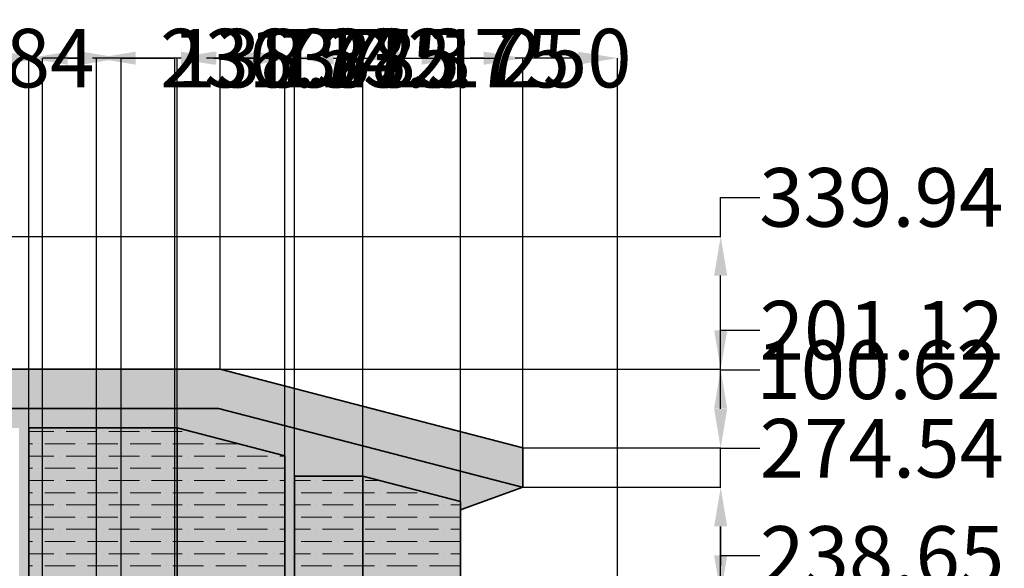
# Model space of a CAD drawing. Units: millimetres. Extents: x -504 to 6314, y 1290 to 4335.
# Tile 9 of 9: x 3796 to 6314, y 2932 to 4335. Entities that reach past the tile are written whole.
import ezdxf

# ---------------------------------------------------------------- set-up
doc = ezdxf.new("R2010")
doc.units = ezdxf.units.MM
doc.header["$MEASUREMENT"] = 0
for name, color, linetype, lineweight in [('A-ANNO-DIMS', 2, 'Continuous', 18), ('A-ELEV', 7, 'Continuous', 35), ('A-ELEV-PATT', 8, 'Continuous', 13)]:
    doc.layers.add(name, color=color, linetype=linetype, lineweight=lineweight)
doc.styles.get("Standard").update_dxf_attribs({"font": 'arial.ttf'})
doc.dimstyles.get("Standard").update_dxf_attribs({"dimtxt": 150, "dimasz": 100, "dimexe": 0.18, "dimexo": 0.0625, "dimgap": 0.09, "dimtad": 0, "dimtih": 1, "dimtoh": 1, "dimdec": 0, "dimzin": 0, "dimdsep": 46, "dimtxsty": 'Standard', "dimcen": 0.09, "dimadec": 0, "dimazin": 0, "dimtfac": 1, "dimtdec": 0, "dimtofl": 0, "dimtmove": 0, "dimatfit": 3, "dimfxl": 1, "dimtolj": 1, "dimtzin": 0, "dimarcsym": 0})

# ---------------------------------------------------------------- blocks, each defined once
blk = doc.blocks.new('*D22')
at = {"layer": 'A-ANNO-DIMS', "color": 0, "lineweight": -2, "transparency": 16777216}
for p, q in [((3324.5, 3780.7), (3324.5, 4237)), ((3424.5, 4236.8), (3651, 4236.8)), ((4208.6, 4236.8), (3982, 4236.8)), ((4308.6, 3440.7), (4308.6, 4237))]:
    blk.add_line(p, q, dxfattribs=at)
at = {"layer": 'A-ANNO-DIMS', "color": 0, "transparency": 16777216}
for points in [[(3424.5, 4253.4), (3424.5, 4220.1), (3324.5, 4236.8)], [(4208.6, 4253.4), (4208.6, 4220.1), (4308.6, 4236.8)]]:
    blk.add_solid(points, dxfattribs=at)
at = {"layer": 'Defpoints', "color": 0, "transparency": 16777216}
for p in [(4308.6, 4236.8), (3324.5, 3780.6), (4308.6, 3440.7)]:
    blk.add_point(p, dxfattribs=at)
at = {"layer": 'A-ANNO-DIMS', "color": 0, "transparency": 16777216, "insert": (3816.5, 4236.8), "char_height": 150, "attachment_point": 5}
blk.add_mtext('\\A1;984', dxfattribs=at)
blk = doc.blocks.new('*D23')
at = {"layer": 'A-ANNO-DIMS', "color": 0, "lineweight": -2, "transparency": 16777216}
for p, q in [((4308.6, 3440.7), (4308.6, 4237)), ((4408.6, 4236.8), (4443.2, 4236.8)), ((4982.9, 4236.8), (4948.3, 4236.8)), ((5082.9, 3239.6), (5082.9, 4237))]:
    blk.add_line(p, q, dxfattribs=at)
at = {"layer": 'A-ANNO-DIMS', "color": 0, "transparency": 16777216}
for points in [[(4408.6, 4253.4), (4408.6, 4220.1), (4308.6, 4236.8)], [(4982.9, 4253.4), (4982.9, 4220.1), (5082.9, 4236.8)]]:
    blk.add_solid(points, dxfattribs=at)
at = {"layer": 'Defpoints', "color": 0, "transparency": 16777216}
for p in [(5082.9, 4236.8), (4308.6, 3440.7), (5082.9, 3239.6)]:
    blk.add_point(p, dxfattribs=at)
at = {"layer": 'A-ANNO-DIMS', "color": 0, "transparency": 16777216, "insert": (4695.7, 4236.8), "char_height": 150, "attachment_point": 5}
blk.add_mtext('\\A1;774.3', dxfattribs=at)
blk = doc.blocks.new('*D24')
at = {"layer": 'A-ANNO-DIMS', "color": 0, "lineweight": -2, "transparency": 16777216}
for p, q in [((5588.8, 3780.6), (5588.8, 3880.6)), ((5588.8, 3880.6), (5688.8, 3880.6)), ((3324.5, 3780.6), (5589, 3780.6)), ((5588.8, 3540.7), (5588.8, 3680.6)), ((4308.6, 3440.7), (5589, 3440.7))]:
    blk.add_line(p, q, dxfattribs=at)
at = {"layer": 'A-ANNO-DIMS', "color": 0, "transparency": 16777216}
for points in [[(5572.1, 3680.6), (5605.5, 3680.6), (5588.8, 3780.6)], [(5572.1, 3540.7), (5605.5, 3540.7), (5588.8, 3440.7)]]:
    blk.add_solid(points, dxfattribs=at)
at = {"layer": 'Defpoints', "color": 0, "transparency": 16777216}
for p in [(3324.5, 3780.6), (5588.8, 3780.6), (4308.6, 3440.7)]:
    blk.add_point(p, dxfattribs=at)
at = {"layer": 'A-ANNO-DIMS', "color": 0, "transparency": 16777216, "insert": (5999.9, 3880.6), "char_height": 150, "attachment_point": 5}
blk.add_mtext('\\A1;339.94', dxfattribs=at)
blk = doc.blocks.new('*D25')
at = {"layer": 'A-ANNO-DIMS', "color": 0, "lineweight": -2, "transparency": 16777216}
for p, q in [((5588.8, 3339.6), (5588.8, 3439.6)), ((5588.8, 3439.6), (5688.8, 3439.6)), ((5082.9, 3239.6), (5589, 3239.6)), ((5081.2, 3138.9), (5589, 3138.9)), ((5588.8, 3038.9), (5588.8, 2938.9))]:
    blk.add_line(p, q, dxfattribs=at)
at = {"layer": 'A-ANNO-DIMS', "color": 0, "transparency": 16777216}
for points in [[(5572.1, 3339.6), (5605.5, 3339.6), (5588.8, 3239.6)], [(5572.1, 3038.9), (5605.5, 3038.9), (5588.8, 3138.9)]]:
    blk.add_solid(points, dxfattribs=at)
at = {"layer": 'Defpoints', "color": 0, "transparency": 16777216}
for p in [(5082.9, 3239.6), (5588.8, 3239.6), (5081.2, 3138.9)]:
    blk.add_point(p, dxfattribs=at)
at = {"layer": 'A-ANNO-DIMS', "color": 0, "transparency": 16777216, "insert": (5992.4, 3439.6), "char_height": 150, "attachment_point": 5}
blk.add_mtext('\\A1;100.62', dxfattribs=at)
blk = doc.blocks.new('*D26')
at = {"layer": 'A-ANNO-DIMS', "color": 0, "lineweight": -2, "transparency": 16777216}
for p, q in [((5588.8, 3440.7), (5588.8, 3540.7)), ((5588.8, 3540.7), (5688.8, 3540.7)), ((4308.6, 3440.7), (5589, 3440.7)), ((5588.8, 3339.6), (5588.8, 3340.7)), ((5082.9, 3239.6), (5589, 3239.6))]:
    blk.add_line(p, q, dxfattribs=at)
at = {"layer": 'A-ANNO-DIMS', "color": 0, "transparency": 16777216}
for points in [[(5572.1, 3340.7), (5605.5, 3340.7), (5588.8, 3440.7)], [(5572.1, 3339.6), (5605.5, 3339.6), (5588.8, 3239.6)]]:
    blk.add_solid(points, dxfattribs=at)
at = {"layer": 'Defpoints', "color": 0, "transparency": 16777216}
for p in [(4308.6, 3440.7), (5588.8, 3440.7), (5082.9, 3239.6)]:
    blk.add_point(p, dxfattribs=at)
at = {"layer": 'A-ANNO-DIMS', "color": 0, "transparency": 16777216, "insert": (6000.8, 3540.7), "char_height": 150, "attachment_point": 5}
blk.add_mtext('\\A1;201.12', dxfattribs=at)
blk = doc.blocks.new('*D27')
at = {"layer": 'A-ANNO-DIMS', "color": 0, "lineweight": -2, "transparency": 16777216}
for p, q in [((5588.8, 3138.9), (5588.8, 3238.9)), ((5588.8, 3238.9), (5688.8, 3238.9)), ((5081.2, 3138.9), (5589, 3138.9)), ((5588.8, 2964.4), (5588.8, 3038.9)), ((4489, 2864.4), (5589, 2864.4))]:
    blk.add_line(p, q, dxfattribs=at)
at = {"layer": 'A-ANNO-DIMS', "color": 0, "transparency": 16777216}
for points in [[(5572.1, 3038.9), (5605.5, 3038.9), (5588.8, 3138.9)], [(5572.1, 2964.4), (5605.5, 2964.4), (5588.8, 2864.4)]]:
    blk.add_solid(points, dxfattribs=at)
at = {"layer": 'Defpoints', "color": 0, "transparency": 16777216}
for p in [(5081.2, 3138.9), (5588.8, 3138.9), (4489, 2864.4)]:
    blk.add_point(p, dxfattribs=at)
at = {"layer": 'A-ANNO-DIMS', "color": 0, "transparency": 16777216, "insert": (6001.2, 3238.9), "char_height": 150, "attachment_point": 5}
blk.add_mtext('\\A1;274.54', dxfattribs=at)
blk = doc.blocks.new('*D28')
at = {"layer": 'A-ANNO-DIMS', "color": 0, "lineweight": -2, "transparency": 16777216}
for p, q in [((-191.2, 3540.7), (-191.2, 3640.7)), ((-191.2, 3640.7), (-91.2, 3640.7)), ((4308.5, 3440.7), (-191.3, 3440.7)), ((4304.4, 3340.7), (-191.3, 3340.7)), ((-191.2, 3240.7), (-191.2, 3140.7))]:
    blk.add_line(p, q, dxfattribs=at)
at = {"layer": 'A-ANNO-DIMS', "color": 0, "transparency": 16777216}
for points in [[(-207.8, 3540.7), (-174.5, 3540.7), (-191.2, 3440.7)], [(-207.8, 3240.7), (-174.5, 3240.7), (-191.2, 3340.7)]]:
    blk.add_solid(points, dxfattribs=at)
at = {"layer": 'Defpoints', "color": 0, "transparency": 16777216}
for p in [(-191.2, 3440.7), (4308.6, 3440.7), (4304.5, 3340.7)]:
    blk.add_point(p, dxfattribs=at)
at = {"layer": 'A-ANNO-DIMS', "color": 0, "transparency": 16777216, "insert": (67.3, 3640.7), "char_height": 150, "attachment_point": 5}
blk.add_mtext('\\A1;100', dxfattribs=at)
blk = doc.blocks.new('*D29')
at = {"layer": 'A-ANNO-DIMS', "color": 0, "lineweight": -2, "transparency": 16777216}
for p, q in [((5588.8, 2864.4), (5588.8, 2964.4)), ((5588.8, 2964.4), (5688.8, 2964.4)), ((4489, 2864.4), (5589, 2864.4)), ((5588.8, 2725.8), (5588.8, 2764.4)), ((4260.1, 2625.8), (5589, 2625.8))]:
    blk.add_line(p, q, dxfattribs=at)
at = {"layer": 'A-ANNO-DIMS', "color": 0, "transparency": 16777216}
for points in [[(5572.1, 2764.4), (5605.5, 2764.4), (5588.8, 2864.4)], [(5572.1, 2725.8), (5605.5, 2725.8), (5588.8, 2625.8)]]:
    blk.add_solid(points, dxfattribs=at)
at = {"layer": 'Defpoints', "color": 0, "transparency": 16777216}
for p in [(4489, 2864.4), (5588.8, 2864.4), (4260, 2625.8)]:
    blk.add_point(p, dxfattribs=at)
at = {"layer": 'A-ANNO-DIMS', "color": 0, "transparency": 16777216, "insert": (6002.1, 2964.4), "char_height": 150, "attachment_point": 5}
blk.add_mtext('\\A1;238.65', dxfattribs=at)
blk = doc.blocks.new('*D44')
at = {"layer": 'A-ANNO-DIMS', "color": 0, "lineweight": -2, "transparency": 16777216}
for p, q in [((4198.6, 3290.7), (4198.6, 4237)), ((4298.6, 4236.8), (4373.6, 4236.8)), ((4473.6, 3219.3), (4473.6, 4237)), ((4473.6, 4236.8), (4573.6, 4236.8))]:
    blk.add_line(p, q, dxfattribs=at)
at = {"layer": 'A-ANNO-DIMS', "color": 0, "transparency": 16777216}
for points in [[(4298.6, 4253.4), (4298.6, 4220.1), (4198.6, 4236.8)], [(4373.6, 4253.4), (4373.6, 4220.1), (4473.6, 4236.8)]]:
    blk.add_solid(points, dxfattribs=at)
at = {"layer": 'Defpoints', "color": 0, "transparency": 16777216}
for p in [(4473.6, 4236.8), (4198.6, 3290.7), (4473.6, 3219.3)]:
    blk.add_point(p, dxfattribs=at)
at = {"layer": 'A-ANNO-DIMS', "color": 0, "transparency": 16777216, "insert": (4741.3, 4236.8), "char_height": 150, "attachment_point": 5}
blk.add_mtext('\\A1;275', dxfattribs=at)
blk = doc.blocks.new('*D45')
at = {"layer": 'A-ANNO-DIMS', "color": 0, "lineweight": -2, "transparency": 16777216}
for p, q in [((4373.6, 4236.8), (4273.6, 4236.8)), ((4473.6, 3219.3), (4473.6, 4237)), ((4498.6, 3167.4), (4498.6, 4237)), ((4598.6, 4236.8), (4698.6, 4236.8))]:
    blk.add_line(p, q, dxfattribs=at)
at = {"layer": 'A-ANNO-DIMS', "color": 0, "transparency": 16777216}
for points in [[(4373.6, 4253.4), (4373.6, 4220.1), (4473.6, 4236.8)], [(4598.6, 4253.4), (4598.6, 4220.1), (4498.6, 4236.8)]]:
    blk.add_solid(points, dxfattribs=at)
at = {"layer": 'Defpoints', "color": 0, "transparency": 16777216}
for p in [(4498.6, 4236.8), (4473.6, 3219.3), (4498.6, 3167.3)]:
    blk.add_point(p, dxfattribs=at)
at = {"layer": 'A-ANNO-DIMS', "color": 0, "transparency": 16777216, "insert": (4808, 4236.8), "char_height": 150, "attachment_point": 5}
blk.add_mtext('\\A1;25', dxfattribs=at)
blk = doc.blocks.new('*D46')
at = {"layer": 'A-ANNO-DIMS', "color": 0, "lineweight": -2, "transparency": 16777216}
for p, q in [((4398.6, 4236.8), (4298.6, 4236.8)), ((4498.6, 3167.4), (4498.6, 4237)), ((4673.6, 3167.4), (4673.6, 4237)), ((4773.6, 4236.8), (4873.6, 4236.8))]:
    blk.add_line(p, q, dxfattribs=at)
at = {"layer": 'A-ANNO-DIMS', "color": 0, "transparency": 16777216}
for points in [[(4398.6, 4253.4), (4398.6, 4220.1), (4498.6, 4236.8)], [(4773.6, 4253.4), (4773.6, 4220.1), (4673.6, 4236.8)]]:
    blk.add_solid(points, dxfattribs=at)
at = {"layer": 'Defpoints', "color": 0, "transparency": 16777216}
for p in [(4673.6, 4236.8), (4498.6, 3167.3), (4673.6, 3167.3)]:
    blk.add_point(p, dxfattribs=at)
at = {"layer": 'A-ANNO-DIMS', "color": 0, "transparency": 16777216, "insert": (5032.9, 4236.8), "char_height": 150, "attachment_point": 5}
blk.add_mtext('\\A1;175', dxfattribs=at)
blk = doc.blocks.new('*D47')
at = {"layer": 'A-ANNO-DIMS', "color": 0, "lineweight": -2, "transparency": 16777216}
for p, q in [((4673.6, 3167.4), (4673.6, 4237)), ((4773.6, 4236.8), (4823.6, 4236.8)), ((4923.6, 3102.4), (4923.6, 4237)), ((4923.6, 4236.8), (5023.6, 4236.8))]:
    blk.add_line(p, q, dxfattribs=at)
at = {"layer": 'A-ANNO-DIMS', "color": 0, "transparency": 16777216}
for points in [[(4773.6, 4253.4), (4773.6, 4220.1), (4673.6, 4236.8)], [(4823.6, 4253.4), (4823.6, 4220.1), (4923.6, 4236.8)]]:
    blk.add_solid(points, dxfattribs=at)
at = {"layer": 'Defpoints', "color": 0, "transparency": 16777216}
for p in [(4923.6, 4236.8), (4673.6, 3167.3), (4923.6, 3102.4)]:
    blk.add_point(p, dxfattribs=at)
at = {"layer": 'A-ANNO-DIMS', "color": 0, "transparency": 16777216, "insert": (5190.5, 4236.8), "char_height": 150, "attachment_point": 5}
blk.add_mtext('\\A1;250', dxfattribs=at)
blk = doc.blocks.new('*D60')
at = {"layer": 'A-ANNO-DIMS', "color": 0, "lineweight": -2, "transparency": 16777216}
for p, q in [((3818.6, 2525.8), (3818.6, 4237)), ((3918.6, 4236.8), (3955.1, 4236.8)), ((4055.1, 2525.8), (4055.1, 4237)), ((4055.1, 4236.8), (4155.1, 4236.8))]:
    blk.add_line(p, q, dxfattribs=at)
at = {"layer": 'A-ANNO-DIMS', "color": 0, "transparency": 16777216}
for points in [[(3918.6, 4253.4), (3918.6, 4220.1), (3818.6, 4236.8)], [(3955.1, 4253.4), (3955.1, 4220.1), (4055.1, 4236.8)]]:
    blk.add_solid(points, dxfattribs=at)
at = {"layer": 'Defpoints', "color": 0, "transparency": 16777216}
for p in [(4055.1, 4236.8), (3818.6, 2525.8), (4055.1, 2525.8)]:
    blk.add_point(p, dxfattribs=at)
at = {"layer": 'A-ANNO-DIMS', "color": 0, "transparency": 16777216, "insert": (4410.2, 4236.8), "char_height": 150, "attachment_point": 5}
blk.add_mtext('\\A1;236.5', dxfattribs=at)
blk = doc.blocks.new('*D61')
at = {"layer": 'A-ANNO-DIMS', "color": 0, "lineweight": -2, "transparency": 16777216}
for p, q in [((3955.1, 4236.8), (3855.1, 4236.8)), ((4055.1, 2525.8), (4055.1, 4237)), ((4192.1, 2525.8), (4192.1, 4237)), ((4292.1, 4236.8), (4392.1, 4236.8))]:
    blk.add_line(p, q, dxfattribs=at)
at = {"layer": 'A-ANNO-DIMS', "color": 0, "transparency": 16777216}
for points in [[(3955.1, 4253.4), (3955.1, 4220.1), (4055.1, 4236.8)], [(4292.1, 4253.4), (4292.1, 4220.1), (4192.1, 4236.8)]]:
    blk.add_solid(points, dxfattribs=at)
at = {"layer": 'Defpoints', "color": 0, "transparency": 16777216}
for p in [(4192.1, 4236.8), (4055.1, 2525.8), (4192.1, 2525.8)]:
    blk.add_point(p, dxfattribs=at)
at = {"layer": 'A-ANNO-DIMS', "color": 0, "transparency": 16777216, "insert": (4550.9, 4236.8), "char_height": 150, "attachment_point": 5}
blk.add_mtext('\\A1;137', dxfattribs=at)
blk = doc.blocks.new('*D62')
at = {"layer": 'A-ANNO-DIMS', "color": 0, "lineweight": -2, "transparency": 16777216}
for p, q in [((4192.1, 2525.8), (4192.1, 4237)), ((4292.1, 4236.8), (4454.1, 4236.8)), ((5224.8, 4236.8), (5062.8, 4236.8)), ((5324.8, 2338.9), (5324.8, 4237))]:
    blk.add_line(p, q, dxfattribs=at)
at = {"layer": 'A-ANNO-DIMS', "color": 0, "transparency": 16777216}
for points in [[(4292.1, 4253.4), (4292.1, 4220.1), (4192.1, 4236.8)], [(5224.8, 4253.4), (5224.8, 4220.1), (5324.8, 4236.8)]]:
    blk.add_solid(points, dxfattribs=at)
at = {"layer": 'Defpoints', "color": 0, "transparency": 16777216}
for p in [(5324.8, 4236.8), (4192.1, 2525.8), (5324.8, 2338.8)]:
    blk.add_point(p, dxfattribs=at)
at = {"layer": 'A-ANNO-DIMS', "color": 0, "transparency": 16777216, "insert": (4758.5, 4236.8), "char_height": 150, "attachment_point": 5}
blk.add_mtext('\\A1;1132.7', dxfattribs=at)
blk = doc.blocks.new('*D66')
at = {"layer": 'A-ANNO-DIMS', "color": 0, "lineweight": -2, "transparency": 16777216}
for p, q in [((3753.7, 4236.8), (3653.7, 4236.8)), ((3853.7, 1932.9), (3853.7, 4237)), ((3992.1, 1982.9), (3992.1, 4237)), ((4092.1, 4236.8), (4192.1, 4236.8))]:
    blk.add_line(p, q, dxfattribs=at)
at = {"layer": 'A-ANNO-DIMS', "color": 0, "transparency": 16777216}
for points in [[(3753.7, 4253.4), (3753.7, 4220.1), (3853.7, 4236.8)], [(4092.1, 4253.4), (4092.1, 4220.1), (3992.1, 4236.8)]]:
    blk.add_solid(points, dxfattribs=at)
at = {"layer": 'Defpoints', "color": 0, "transparency": 16777216}
for p in [(3992.1, 4236.8), (3992.1, 1982.8), (3853.7, 1932.8)]:
    blk.add_point(p, dxfattribs=at)
at = {"layer": 'A-ANNO-DIMS', "color": 0, "transparency": 16777216, "insert": (4496.6, 4236.8), "char_height": 150, "attachment_point": 5}
blk.add_mtext('\\A1;138.38', dxfattribs=at)

msp = doc.modelspace()

# ---------------------------------------------------------------- hatches: boundary and pattern name
at = {"layer": 'A-ELEV-PATT'}
msp.add_hatch(color=256, dxfattribs=at).paths.add_polyline_path([(4308.57, 3440.687), (3929.687, 3440.687), (3407.797, 3440.687), (1778.718, 3440.687), (1828.718, 3340.687), (3407.797, 3340.687), (3929.687, 3340.687), (4304.463, 3340.687), (5081.168, 3138.941), (5082.876, 3139.564), (5082.876, 3239.564)])
h = msp.add_hatch(dxfattribs=at)
h.set_pattern_fill('AR-CONC', color=256, scale=10, style=0)
h.set_pattern_definition([(50, (0, 0), (71.726, -6.2752), [7.5, -82.5]), (355, (0, 0), (-13.8751, 75.2192), [6, -66]), (100.4514, (5.98, -0.52), (57.8509, 68.944), [6.374, -70.1142]), (46.1842, (0, 20), (106.7241, -16.5519), [11.25, -123.75]), (96.6356, (8.89, 18.62), (93.4662, 97.4119), [9.561, -105.1714]), (351.1842, (0, 20), (93.4662, 97.4119), [9, -99]), (21, (10, 15), (59.6907, -40.2619), [7.5, -82.5]), (326, (10, 15), (24.3315, 72.515), [6, -66]), (71.4514, (14.974, 11.645), (84.0222, 32.2531), [6.374, -70.1142]), (37.5, (0, 0), (1.21599, 33.28939), [0, -65.2, 0, -67, 0, -66.25]), (7.5, (0, 0), (26.30695, 39.44117), [0, -38.2, 0, -63.7, 0, -25.25]), (327.5, (-22.3, 0), (53.38224, -2.25549), [0, -25, 0, -78, 0, -103.5]), (317.5, (-32.3, 0), (58.3186, 10.0105), [0, -32.5, 0, -51.8, 0, -73.5])])
h.paths.add_polyline_path([(4308.57, 3440.687), (3929.687, 3440.687), (3407.797, 3440.687), (1778.718, 3440.687), (1828.718, 3340.687), (3407.797, 3340.687), (3929.687, 3340.687), (4304.463, 3340.687), (5081.168, 3138.941), (5082.876, 3139.564), (5082.876, 3239.564)])
h.paths.add_polyline_path([(4260.021, 2625.758), (3929.687, 2625.758), (3407.797, 2625.758), (2186.182, 2625.758), (2223.682, 2550.758), (3407.797, 2550.758), (3929.687, 2550.758), (4250.093, 2550.758), (5324.792, 2261.16), (5324.792, 2338.836)])
h = msp.add_hatch(color=256, dxfattribs=at)
h.paths.add_polyline_path([(4304.463, 3340.687), (3929.687, 3340.687), (3407.797, 3340.687), (1828.718, 3340.687), (1853.718, 3290.687), (1976.702, 3290.687), (2309.166, 2625.758), (2353.888, 2625.758), (2021.423, 3290.687), (2963.634, 3290.687), (2963.634, 3265.687), (3407.797, 3265.687), (3768.634, 3265.687), (3768.634, 3290.687), (3793.634, 3290.687), (3793.634, 2625.758), (3818.634, 2625.758), (3818.634, 3290.687), (3929.687, 3290.687), (4198.634, 3290.687), (4473.634, 3219.257), (4473.634, 2568.197), (4498.634, 2561.46), (4498.634, 3167.307), (4673.634, 3167.307), (4923.634, 3102.371), (4923.634, 3081.487), (5081.168, 3138.941)])
h.paths.add_polyline_path([(3768.634, 3240.687), (3407.797, 3240.687), (2963.634, 3240.687), (2963.634, 3290.687), (2913.634, 3290.687), (2913.634, 2625.758), (2963.634, 2625.758), (2963.634, 3215.687), (3407.797, 3215.687), (3768.634, 3215.687)], flags=17)
h = msp.add_hatch(color=256, dxfattribs=at)
h.paths.add_polyline_path([(2888.634, 3290.687), (2021.423, 3290.687), (2353.888, 2625.758), (2888.634, 2625.758)])
h.paths.add_polyline_path([(4198.634, 3290.687), (3929.687, 3290.687), (3818.634, 3290.687), (3818.634, 2625.758), (3929.687, 2625.758), (4198.634, 2625.758)])
h.paths.add_polyline_path([(4473.634, 3219.257), (4198.634, 3290.687), (4198.634, 2625.758), (4260.021, 2625.758), (4473.634, 2568.197)])
h.paths.add_polyline_path([(4673.634, 3167.307), (4498.634, 3167.307), (4498.634, 2561.46), (4673.634, 2514.303)])
h.paths.add_polyline_path([(4923.634, 3102.371), (4673.634, 3167.307), (4673.634, 2514.303), (4923.634, 2446.935)])
h = msp.add_hatch(dxfattribs=at)
h.set_pattern_fill('ANSI36', color=256, scale=250, angle=135, style=0)
h.paths.add_polyline_path([(2888.634, 3290.687), (2021.423, 3290.687), (2231.996, 2869.543), (2888.634, 2868.048)])
h.paths.add_polyline_path([(4198.634, 3290.687), (3929.687, 3290.687), (3818.634, 3290.687), (3818.634, 2865.931), (4198.634, 2865.066)])
h.paths.add_polyline_path([(4473.634, 3219.257), (4198.634, 3290.687), (4198.634, 2865.066), (4473.634, 2864.44)])
h.paths.add_polyline_path([(4923.634, 3102.371), (4673.634, 3167.307), (4673.634, 2814.647), (4923.634, 2747.28)])
h.paths.add_polyline_path([(4673.634, 3167.307), (4498.634, 3167.307), (4498.634, 2861.804), (4673.634, 2814.647)])
h.paths.add_polyline_path([(4673.634, 2814.647), (4498.634, 2861.804), (4498.634, 2561.46), (4673.634, 2514.303)])
h.paths.add_polyline_path([(4923.634, 2747.28), (4673.634, 2814.647), (4673.634, 2514.303), (4923.634, 2446.935)])
h.paths.add_polyline_path([(4473.634, 2864.44), (4198.634, 2865.066), (4198.634, 2625.758), (4260.021, 2625.758), (4473.634, 2568.197)])
h.paths.add_polyline_path([(4198.634, 2865.066), (3818.634, 2865.931), (3818.634, 2625.758), (3929.687, 2625.758), (4198.634, 2625.758)])
h.paths.add_polyline_path([(2888.634, 2868.048), (2231.996, 2869.543), (2353.888, 2625.758), (2888.634, 2625.758)])

# ---------------------------------------------------------------- linework, layer by layer
at = {"layer": 'A-ELEV'}
for p, q in [((3407.797, 3440.687), (3929.687, 3440.687)), ((3929.687, 3440.687), (4308.57, 3440.687)), ((4308.57, 3440.687), (5082.876, 3239.564)), ((3407.797, 3340.687), (3929.687, 3340.687)), ((3929.687, 3340.687), (4304.463, 3340.687)), ((4304.463, 3340.687), (5081.168, 3138.941)), ((3818.634, 3290.687), (3818.634, 2625.758)), ((3818.634, 3290.687), (3929.687, 3290.687)), ((3929.687, 3290.687), (4198.634, 3290.687)), ((4198.634, 3290.687), (4473.634, 3219.257)), ((4198.634, 3290.687), (4198.634, 2625.758)), ((5082.876, 3239.564), (5082.876, 3139.564)), ((4473.634, 3219.257), (4473.634, 2568.197)), ((4498.634, 3167.307), (4498.634, 2561.46)), ((4673.634, 3167.307), (4498.634, 3167.307)), ((4673.634, 3167.307), (4673.634, 2514.303)), ((4673.634, 3167.307), (4923.634, 3102.371)), ((5082.876, 3139.564), (4923.634, 3081.487)), ((4923.634, 3102.371), (4923.634, 2446.935))]:
    msp.add_line(p, q, dxfattribs=at)

# ---------------------------------------------------------------- dimensions: what is measured, and where the dimension line sits
at = {"layer": 'A-ANNO-DIMS'}
for base, p1, p2, override, picture, middle in [((4308.57, 4236.781), (3324.48, 3780.626), (4308.57, 3440.687), {"dimdec": 0, "dimlfac": 1, "dimrnd": 0, "dimzin": 0, "dimdsep": 46, "dimlunit": 2}, '*D22', (3816.525, 4236.781)), ((3992.087, 4236.781), (3853.708, 1932.831), (3992.087, 1982.831), {"dimdec": 2, "dimlfac": 1, "dimrnd": 0, "dimzin": 0, "dimdsep": 46, "dimlunit": 2}, '*D66', (4496.628, 4236.781)), ((4055.138, 4236.781), (3818.634, 2525.758), (4055.138, 2525.758), {"dimdec": 1, "dimlfac": 1, "dimrnd": 0, "dimzin": 0, "dimdsep": 46, "dimlunit": 2}, '*D60', (4410.156, 4236.781)), ((4192.131, 4236.781), (4055.138, 2525.758), (4192.131, 2525.758), {"dimdec": 0, "dimlfac": 1, "dimrnd": 0, "dimzin": 0, "dimdsep": 46, "dimlunit": 2}, '*D61', (4550.867, 4236.781)), ((5324.792, 4236.781), (4192.131, 2525.758), (5324.792, 2338.836), {"dimdec": 1, "dimlfac": 1, "dimrnd": 0, "dimzin": 0, "dimdsep": 46, "dimlunit": 2}, '*D62', (4758.461, 4236.781)), ((4473.634, 4236.781), (4198.634, 3290.687), (4473.634, 3219.257), {"dimdec": 0, "dimlfac": 1, "dimrnd": 0, "dimzin": 0, "dimdsep": 46, "dimlunit": 2}, '*D44', (4741.271, 4236.781)), ((4498.634, 4236.781), (4473.634, 3219.257), (4498.634, 3167.307), {"dimdec": 0, "dimlfac": 1, "dimrnd": 0, "dimzin": 0, "dimdsep": 46, "dimlunit": 2}, '*D45', (4808.001, 4236.781)), ((4673.634, 4236.781), (4498.634, 3167.307), (4673.634, 3167.307), {"dimdec": 0, "dimlfac": 1, "dimrnd": 0, "dimzin": 0, "dimdsep": 46, "dimlunit": 2}, '*D46', (5032.932, 4236.781)), ((5082.876, 4236.781), (4308.57, 3440.687), (5082.876, 3239.564), {"dimdec": 1, "dimlfac": 1, "dimrnd": 0, "dimzin": 0, "dimdsep": 46, "dimlunit": 2}, '*D23', (4695.723, 4236.781)), ((4923.634, 4236.781), (4673.634, 3167.307), (4923.634, 3102.371), {"dimdec": 0, "dimlfac": 1, "dimrnd": 0, "dimzin": 0, "dimdsep": 46, "dimlunit": 2}, '*D47', (5190.453, 4236.781))]:
    dim = msp.add_linear_dim(base=base, p1=p1, p2=p2, dimstyle='Standard', override=override, dxfattribs=at)
    dim.commit()
    dim.dimension.update_dxf_attribs({"geometry": picture, "text_midpoint": middle})
for base, p1, p2, override, picture, middle in [((5588.792, 3780.626), (4308.57, 3440.687), (3324.48, 3780.626), {"dimdec": 2, "dimlfac": 1, "dimrnd": 0, "dimzin": 0, "dimdsep": 46, "dimlunit": 2}, '*D24', (5999.881, 3880.626)), ((-191.165, 3440.687), (4304.463, 3340.687), (4308.57, 3440.687), {"dimdec": 0, "dimlfac": 1, "dimrnd": 0, "dimzin": 0, "dimdsep": 46, "dimlunit": 2}, '*D28', (67.315, 3640.687)), ((5588.792, 3440.687), (5082.876, 3239.564), (4308.57, 3440.687), {"dimdec": 2, "dimlfac": 1, "dimrnd": 0, "dimzin": 0, "dimdsep": 46, "dimlunit": 2}, '*D26', (6000.751, 3540.687)), ((5588.792, 3239.564), (5081.168, 3138.941), (5082.876, 3239.564), {"dimdec": 2, "dimlfac": 1, "dimrnd": 0, "dimzin": 0, "dimdsep": 46, "dimlunit": 2}, '*D25', (5992.412, 3439.564)), ((5588.7921, 3138.9408), (4488.9803, 2864.4056), (5081.1676, 3138.9408), {"dimdec": 2, "dimlfac": 1, "dimrnd": 0, "dimzin": 0, "dimdsep": 46, "dimlunit": 2}, '*D27', (6001.2116, 3238.9408)), ((5588.792, 2864.406), (4260.021, 2625.758), (4488.98, 2864.406), {"dimdec": 2, "dimlfac": 1, "dimrnd": 0, "dimzin": 0, "dimdsep": 46, "dimlunit": 2}, '*D29', (6002.081, 2964.406))]:
    dim = msp.add_linear_dim(base=base, p1=p1, p2=p2, angle=90, dimstyle='Standard', override=override, dxfattribs=at)
    dim.commit()
    dim.dimension.update_dxf_attribs({"geometry": picture, "text_midpoint": middle})

doc.saveas('drawing.dxf')
